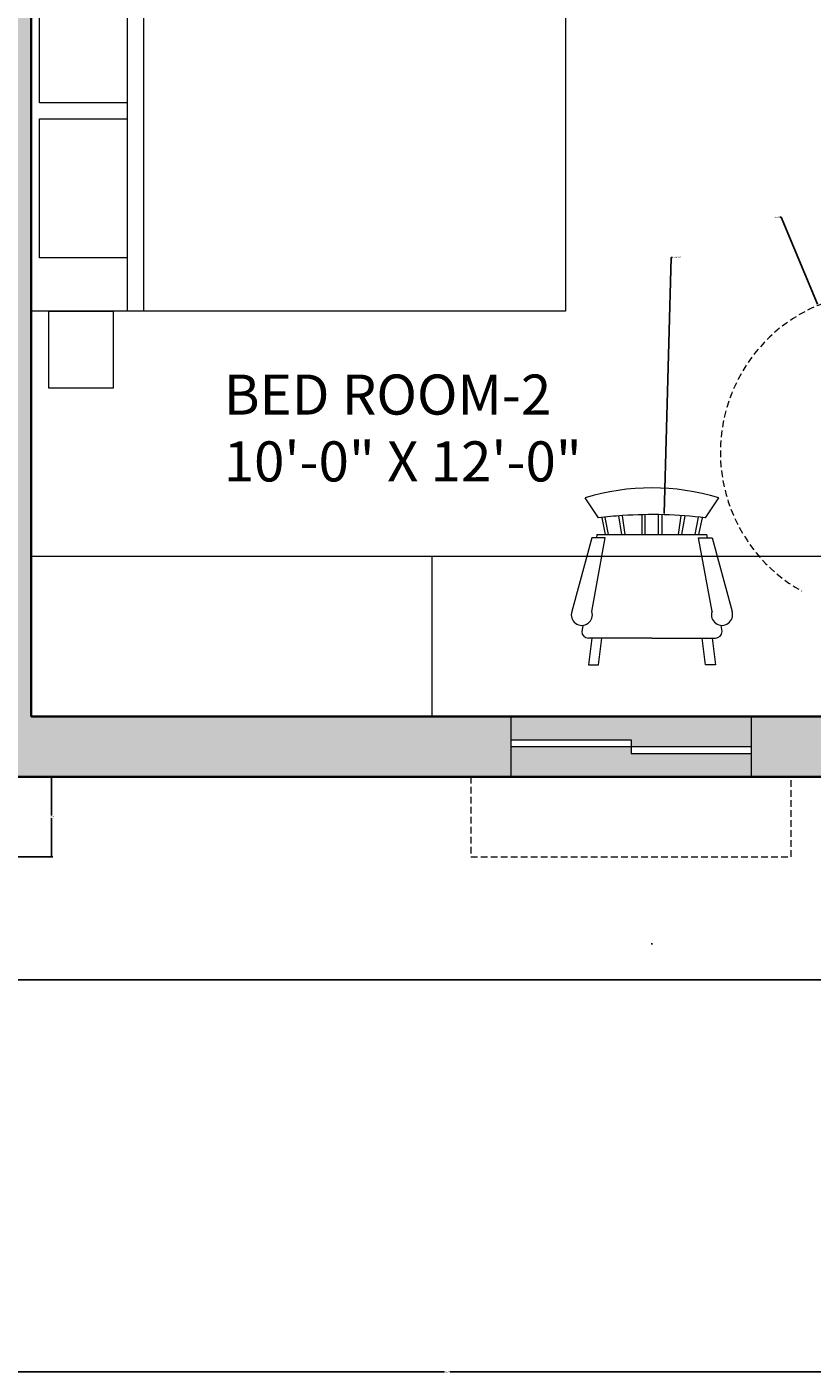
# Model space of a CAD drawing. Units: inches. Extents: x 1693 to 2974, y 2201 to 2965.
# Tile 8 of 24: x 1976 to 2093, y 2201 to 2402. Entities that reach past the tile are written whole.
import ezdxf

# ---------------------------------------------------------------- set-up
doc = ezdxf.new("R2010")
doc.units = ezdxf.units.IN
doc.header["$LTSCALE"] = 2
doc.header["$MEASUREMENT"] = 0
doc.linetypes.add('HIDDEN', pattern=[0.375, 0.25, -0.125])
for name, color, linetype, lineweight in [('A-ANNO-DIMS', 2, 'Continuous', 18), ('A-AREA-IDEN', 7, 'Continuous', 18), ('A-DOOR-SWNG', 3, 'HIDDEN', 13), ('A-FLOR-CASE', 32, 'Continuous', 18), ('A-FURN', 8, 'Continuous', 18), ('A-GLAZ', 4, 'Continuous', 18), ('A-GLAZ-OVHD', 8, 'HIDDEN', 13), ('A-WALL', 7, 'Continuous', 35)]:
    doc.layers.add(name, color=color, linetype=linetype, lineweight=lineweight)
doc.layers.add('A-GLAZ-PATT', color=141, linetype='Continuous', lineweight=13, true_color=0xadddf7)
doc.layers.add('A-WALL-PATT', color=251, linetype='Continuous', lineweight=13, true_color=0x636466)
doc.styles.get("Standard").update_dxf_attribs({"font": 'arial.ttf'})
doc.dimstyles.get("Standard").update_dxf_attribs({"dimtxt": 0.18, "dimasz": 0.18, "dimexe": 0.18, "dimexo": 0.0625, "dimgap": 0.09, "dimtad": 0, "dimtih": 1, "dimtoh": 1, "dimdec": 1, "dimzin": 0, "dimdsep": 46, "dimlunit": 3, "dimtxsty": 'Standard', "dimcen": 0.09, "dimadec": 0, "dimazin": 0, "dimtfac": 1, "dimtdec": 1, "dimtofl": 0, "dimtmove": 0, "dimatfit": 3, "dimfxl": 1, "dimtolj": 1, "dimtzin": 0, "dimarcsym": 0})

# ---------------------------------------------------------------- blocks, each defined once
blk = doc.blocks.new('Chair - Rocking')
for p, q in [((-8, -4.5), (-10, -1.5)), ((8, -4.5), (10, -1.5)), ((-7.5, -4.5), (-7, -7)), ((-6.5, -7), (-7.02225, -4.43)), ((-4.5, -7), (-4.96674, -4.19951)), ((-4, -7), (-4.40532, -4.16272)), ((-1.5, -4.05012), (-1.5, -7)), ((-1, -7), (-1, -4.05012)), ((1, -7), (1, -4.04655)), ((1.5, -4.05012), (1.5, -7)), ((4, -7), (4.40187, -4.18694)), ((4.5, -7), (4.96761, -4.19437)), ((6.5, -7), (7, -4.4057)), ((7.5, -4.5), (7, -7)), ((-9, -7.5), (-12, -18.49999)), ((-7, -7.5), (-9, -7.5)), ((-9, -18.49999), (-7, -7.5)), ((-8.23428, -6.99939), (-8.3093, -7.47958)), ((-8.23041, -7), (8.23915, -7)), ((7, -7.5), (9, -7.5)), ((9, -18.49999), (7, -7.5)), ((8.31071, -7.48854), (8.23449, -7.00073)), ((9, -7.5), (12, -18.49999)), ((-10.36644, -20.64523), (-10.5, -21.49999)), ((10.5, -21.49999), (10.3575, -20.58798)), ((-9, -22.49999), (-9.5, -26.49999)), ((0, -22.49999), (-9.5, -22.49999)), ((-8, -26.49999), (-7.5, -22.49999)), ((0, -22.49999), (9.5, -22.49999)), ((8, -26.49999), (7.5, -22.49999)), ((9, -22.49999), (9.5, -26.49999)), ((-9.5, -26.49999), (-8, -26.49999)), ((9.5, -26.49999), (8, -26.49999))]:
    blk.add_line(p, q)
for centre, radius, start, end in [((0, -34.08333), 34.08333, 72.93847, 107.0615), ((0, -68.25004), 64.25, 82.84733, 93.92211), ((0, -68.25004), 64.25, 93.92211, 97.15267), ((-10.5, -18.99999), 1.58114, 161.5651, 18.43495), ((10.5, -18.99999), 1.58114, 161.5651, 18.43495), ((-9.5, -21.49999), 1, 180, 270), ((9.5, -21.49999), 1, 270, 0)]:
    blk.add_arc(centre, radius, start, end)
blk = doc.blocks.new('Bed - Queen')
for p, q in [((0, -80.00003), (0, 0)), ((0, 0), (59.99999, 0)), ((59.99999, 0), (59.99999, -80.00003)), ((7.99999, -1.2), (28.79998, -1.2)), ((7.99999, -14.4), (7.99999, -1.2)), ((28.79998, -1.2), (28.79998, -14.4)), ((31.19999, -1.2), (51.99999, -1.2)), ((31.19999, -14.4), (31.19999, -1.2)), ((51.99999, -1.2), (51.99999, -16.4)), ((0, -14.4), (44.8, -14.4)), ((59.99999, -29.6), (44.8, -14.4)), ((44.8, -14.4), (44.8, -29.6)), ((44.8, -16.8), (0, -16.8)), ((51.99999, -16.4), (46.79936, -16.4)), ((44.8, -29.6), (59.99999, -29.6)), ((59.99999, -80.00003), (0, -80.00003))]:
    blk.add_line(p, q)
blk = doc.blocks.new('NIGHTSTAND')
at = {"ltscale": 2}
blk.add_lwpolyline([(11.51, 0), (0, 0), (0, 9.62), (11.51, 9.62)], close=True, dxfattribs=at)
blk = doc.blocks.new('WINDOW-HOOD-48IN')
at = {"ltscale": 2}
for p, q in [((12, 48), (0, 48)), ((0, 48), (0, 6)), ((12, 42), (12, 48)), ((0, 6), (0, 0)), ((0, 0), (12, 0))]:
    blk.add_line(p, q, dxfattribs=at)
blk = doc.blocks.new('*D52')
at = {"layer": 'A-ANNO-DIMS', "color": 0, "lineweight": -2, "ltscale": 2, "transparency": 16777216}
for p, q in [((1972.14, 2289.84), (1979.46, 2289.84)), ((1979.28, 2289.66), (1979.28, 2284.03)), ((1979.28, 2278.02), (1979.28, 2283.66)), ((1972.14, 2277.84), (1979.46, 2277.84))]:
    blk.add_line(p, q, dxfattribs=at)
at = {"layer": 'A-ANNO-DIMS', "color": 0, "ltscale": 2, "transparency": 16777216}
for points in [[(1979.25, 2289.66), (1979.31, 2289.66), (1979.28, 2289.84)], [(1979.25, 2278.02), (1979.31, 2278.02), (1979.28, 2277.84)]]:
    blk.add_solid(points, dxfattribs=at)
at = {"layer": 'Defpoints', "color": 0, "ltscale": 2, "transparency": 16777216}
for p in [(1972.08, 2289.84), (1979.28, 2289.84), (1972.08, 2277.84)]:
    blk.add_point(p, dxfattribs=at)
at = {"layer": 'A-ANNO-DIMS', "color": 0, "ltscale": 2, "transparency": 16777216, "insert": (1979.28, 2283.84), "char_height": 0.18, "attachment_point": 5}
blk.add_mtext('\\A1;12 TYP.', dxfattribs=at)
blk = doc.blocks.new('*D82')
at = {"layer": 'A-ANNO-DIMS', "color": 0, "lineweight": -2, "ltscale": 2, "transparency": 16777216}
for p, q in [((2615.67, 2906.08), (1693.46, 2906.08)), ((1693.64, 2905.9), (1693.64, 2582.94)), ((1693.64, 2259.62), (1693.64, 2582.58)), ((2096.17, 2259.44), (1693.46, 2259.44))]:
    blk.add_line(p, q, dxfattribs=at)
at = {"layer": 'A-ANNO-DIMS', "color": 0, "ltscale": 2, "transparency": 16777216}
for points in [[(1693.61, 2905.9), (1693.67, 2905.9), (1693.64, 2906.08)], [(1693.61, 2259.62), (1693.67, 2259.62), (1693.64, 2259.44)]]:
    blk.add_solid(points, dxfattribs=at)
at = {"layer": 'Defpoints', "color": 0, "ltscale": 2, "transparency": 16777216}
for p in [(1693.64, 2906.08), (2615.74, 2906.08), (2096.24, 2259.44)]:
    blk.add_point(p, dxfattribs=at)
at = {"layer": 'A-ANNO-DIMS', "color": 0, "ltscale": 2, "transparency": 16777216, "insert": (1693.64, 2582.76), "char_height": 0.18, "attachment_point": 5}
blk.add_mtext('\\A1;646.6', dxfattribs=at)
blk = doc.blocks.new('*D83')
at = {"layer": 'A-ANNO-DIMS', "color": 0, "lineweight": -2, "ltscale": 2, "transparency": 16777216}
for p, q in [((1782.74, 2289.78), (1782.74, 2200.56)), ((2294.24, 2289.78), (2294.24, 2200.56)), ((1782.92, 2200.74), (2038.09, 2200.74)), ((2294.06, 2200.74), (2038.88, 2200.74))]:
    blk.add_line(p, q, dxfattribs=at)
at = {"layer": 'A-ANNO-DIMS', "color": 0, "ltscale": 2, "transparency": 16777216}
for points in [[(1782.92, 2200.77), (1782.92, 2200.71), (1782.74, 2200.74)], [(2294.06, 2200.77), (2294.06, 2200.71), (2294.24, 2200.74)]]:
    blk.add_solid(points, dxfattribs=at)
at = {"layer": 'Defpoints', "color": 0, "ltscale": 2, "transparency": 16777216}
for p in [(1782.74, 2289.84), (2294.24, 2289.84), (2294.24, 2200.74)]:
    blk.add_point(p, dxfattribs=at)
at = {"layer": 'A-ANNO-DIMS', "color": 0, "ltscale": 2, "transparency": 16777216, "insert": (2038.49, 2200.74), "char_height": 0.18, "attachment_point": 5}
blk.add_mtext('\\A1;511.5', dxfattribs=at)
blk = doc.blocks.new('*D126')
at = {"layer": 'A-ANNO-DIMS', "color": 0, "lineweight": -2, "ltscale": 2, "transparency": 16777216}
for p, q in [((2088.31, 2373.6), (2088.49, 2373.6)), ((2088.49, 2373.6), (2093.95, 2360.58)), ((2103.15, 2338.43), (2103.33, 2338.43)), ((2103.24, 2338.34), (2103.24, 2338.52))]:
    blk.add_line(p, q, dxfattribs=at)
at = {"layer": 'A-ANNO-DIMS', "color": 0, "ltscale": 2, "transparency": 16777216}
blk.add_solid([(2093.98, 2360.59), (2093.93, 2360.57), (2094.02, 2360.41)], dxfattribs=at)
at = {"layer": 'Defpoints', "color": 0, "ltscale": 2, "transparency": 16777216}
for p in [(2094.02, 2360.41), (2103.24, 2338.43)]:
    blk.add_point(p, dxfattribs=at)
at = {"layer": 'A-ANNO-DIMS', "color": 0, "ltscale": 2, "transparency": 16777216, "insert": (2087.83, 2373.6), "char_height": 0.18, "attachment_point": 5}
blk.add_mtext('\\A1;R23.84', dxfattribs=at)
blk = doc.blocks.new('*D129')
at = {"layer": 'A-ANNO-DIMS', "color": 0, "lineweight": -2, "ltscale": 2, "transparency": 16777216}
for p, q in [((2072.05, 2367.59), (2070.97, 2329.24)), ((2072.23, 2367.59), (2072.05, 2367.59)), ((2069.06, 2264.83), (2069.24, 2264.83)), ((2069.15, 2264.74), (2069.15, 2264.92))]:
    blk.add_line(p, q, dxfattribs=at)
at = {"layer": 'A-ANNO-DIMS', "color": 0, "ltscale": 2, "transparency": 16777216}
blk.add_solid([(2070.94, 2329.24), (2071, 2329.24), (2070.96, 2329.06)], dxfattribs=at)
at = {"layer": 'Defpoints', "color": 0, "ltscale": 2, "transparency": 16777216}
for p in [(2070.96, 2329.06), (2069.15, 2264.83)]:
    blk.add_point(p, dxfattribs=at)
at = {"layer": 'A-ANNO-DIMS', "color": 0, "ltscale": 2, "transparency": 16777216, "insert": (2072.91, 2367.59), "char_height": 0.18, "attachment_point": 5}
blk.add_mtext('\\A1;4X R64.25', dxfattribs=at)

msp = doc.modelspace()

# ---------------------------------------------------------------- hatches: boundary and pattern name
at = {"layer": 'A-GLAZ-PATT', "ltscale": 2}
h = msp.add_hatch(color=256, dxfattribs=at)
h.dxf.hatch_style = 1
h.paths.add_polyline_path([(2656.9702, 2338.2547), (2632.9702, 2338.2547), (2632.9702, 2339.2547), (2608.9702, 2339.2547), (2608.9702, 2334.7547), (2656.9702, 2334.7547)])
h.paths.add_polyline_path([(2656.9702, 2343.7547), (2608.9702, 2343.7547), (2608.9702, 2340.2547), (2632.9702, 2340.2547), (2632.9702, 2339.2547), (2656.9702, 2339.2547)])
h.paths.add_polyline_path([(2775.7544, 2338.2547), (2751.7544, 2338.2547), (2751.7544, 2334.7547), (2775.7544, 2334.7547)])
h.paths.add_polyline_path([(2775.7544, 2343.7547), (2751.7544, 2343.7547), (2751.7544, 2340.2547), (2775.7544, 2340.2547)])
h.paths.add_polyline_path([(2897.7363, 2568.7999), (2893.2363, 2568.7999), (2893.2363, 2520.7999), (2896.7363, 2520.7999), (2896.7363, 2544.7999), (2897.7363, 2544.7999)])
h.paths.add_polyline_path([(2902.2363, 2568.7999), (2898.7363, 2568.7999), (2898.7363, 2544.7999), (2897.7363, 2544.7999), (2897.7363, 2520.7999), (2902.2363, 2520.7999)])
h.paths.add_polyline_path([(2902.2363, 2637.7547), (2898.7363, 2637.7547), (2898.7363, 2613.7547), (2902.2363, 2613.7547)])
h.paths.add_polyline_path([(2896.7363, 2637.7547), (2893.2363, 2637.7547), (2893.2363, 2613.7547), (2896.7363, 2613.7547)])
h.paths.add_polyline_path([(2902.2363, 2748.903), (2899.0477, 2748.903), (2899.0477, 2724.903), (2898.0477, 2724.903), (2898.0477, 2700.903), (2902.2363, 2700.903)])
h.paths.add_polyline_path([(2898.0477, 2748.903), (2893.2363, 2748.903), (2893.2363, 2700.903), (2897.0477, 2700.903), (2897.0477, 2724.903), (2898.0477, 2724.903)])
h.paths.add_polyline_path([(2851.2363, 2846.2547), (2803.2363, 2846.2547), (2803.2363, 2842.7547), (2827.2363, 2842.7547), (2827.2363, 2841.7547), (2851.2363, 2841.7547)])
h.paths.add_polyline_path([(2851.2363, 2840.7547), (2827.2363, 2840.7547), (2827.2363, 2841.7547), (2803.2363, 2841.7547), (2803.2363, 2837.2547), (2851.2363, 2837.2547)])
h.paths.add_polyline_path([(2578.2363, 2846.2547), (2530.2363, 2846.2547), (2530.2363, 2842.7547), (2554.2363, 2842.7547), (2554.2363, 2841.7547), (2578.2363, 2841.7547)])
h.paths.add_polyline_path([(2578.2363, 2840.7547), (2554.2363, 2840.7547), (2554.2363, 2841.7547), (2530.2363, 2841.7547), (2530.2363, 2837.2547), (2578.2363, 2837.2547)])
h.paths.add_polyline_path([(2732.7363, 2812.7547), (2705.1363, 2812.7547), (2705.1363, 2811.7547), (2676.3363, 2811.7547), (2676.3363, 2812.7547), (2648.7363, 2812.7547), (2648.7363, 2808.2547), (2732.7363, 2808.2547)])
h.paths.add_polyline_path([(2732.7363, 2817.2547), (2648.7363, 2817.2547), (2648.7363, 2813.7547), (2676.3363, 2813.7547), (2676.3363, 2812.7547), (2705.1363, 2812.7547), (2705.1363, 2813.7547), (2732.7363, 2813.7547)])
h.paths.add_polyline_path([(2488.2363, 2695.8203), (2484.7878, 2695.8203), (2484.7878, 2671.8203), (2488.2363, 2671.8203)])
h.paths.add_polyline_path([(2482.7878, 2695.8203), (2479.2363, 2695.8203), (2479.2363, 2671.8203), (2482.7878, 2671.8203)])
h.paths.add_polyline_path([(2488.2363, 2572.4371), (2484.7363, 2572.4371), (2484.7363, 2541.4371), (2483.7363, 2541.4371), (2483.7363, 2512.4371), (2488.2363, 2512.4371)])
h.paths.add_polyline_path([(2482.7363, 2541.4371), (2483.7363, 2541.4371), (2483.7363, 2572.4371), (2479.2363, 2572.4371), (2479.2363, 2512.4371), (2482.7363, 2512.4371)])
h.paths.add_polyline_path([(2248.9863, 2706.8449), (2190.9863, 2706.8449), (2190.9863, 2703.3449), (2219.9863, 2703.3449), (2219.9863, 2702.3449), (2248.9863, 2702.3449)])
h.paths.add_polyline_path([(2248.9863, 2701.3449), (2219.9863, 2701.3449), (2219.9863, 2702.3449), (2190.9863, 2702.3449), (2190.9863, 2697.8449), (2248.9863, 2697.8449)])
h.paths.add_polyline_path([(2151.9207, 2293.3449), (2127.9207, 2293.3449), (2127.9207, 2289.8449), (2151.9207, 2289.8449)])
h.paths.add_polyline_path([(2151.9207, 2298.8449), (2127.9207, 2298.8449), (2127.9207, 2295.3449), (2151.9207, 2295.3449)])
h.paths.add_polyline_path([(2084.023, 2293.3449), (2066.023, 2293.3449), (2066.023, 2294.3449), (2048.023, 2294.3449), (2048.023, 2289.8449), (2084.023, 2289.8449)])
h.paths.add_polyline_path([(2084.023, 2298.8449), (2048.023, 2298.8449), (2048.023, 2295.3449), (2066.023, 2295.3449), (2066.023, 2294.3449), (2084.023, 2294.3449)])
h.paths.add_polyline_path([(1966.0781, 2293.3449), (1948.0781, 2293.3449), (1948.0781, 2294.3449), (1930.0781, 2294.3449), (1930.0781, 2289.8449), (1966.0781, 2289.8449)])
h.paths.add_polyline_path([(1966.0781, 2298.8449), (1930.0781, 2298.8449), (1930.0781, 2295.3449), (1948.0781, 2295.3449), (1948.0781, 2294.3449), (1966.0781, 2294.3449)])
h.paths.add_polyline_path([(1787.2363, 2403.1922), (1782.7363, 2403.1922), (1782.7363, 2355.1922), (1786.2363, 2355.1922), (1786.2363, 2379.1922), (1787.2363, 2379.1922)])
h.paths.add_polyline_path([(1791.7363, 2403.1922), (1788.2363, 2403.1922), (1788.2363, 2379.1922), (1787.2363, 2379.1922), (1787.2363, 2355.1922), (1791.7363, 2355.1922)])
h.paths.add_polyline_path([(1786.2363, 2477.5455), (1782.7363, 2477.5455), (1782.7363, 2453.5455), (1786.2363, 2453.5455)])
h.paths.add_polyline_path([(1791.7363, 2477.5455), (1788.2363, 2477.5455), (1788.2363, 2453.5455), (1791.7363, 2453.5455)])
h.paths.add_polyline_path([(1786.2363, 2621.6433), (1782.7363, 2621.6433), (1782.7363, 2585.6433), (1786.2363, 2585.6433)])
h.paths.add_polyline_path([(1791.7363, 2621.6433), (1788.2363, 2621.6433), (1788.2363, 2585.6433), (1791.7363, 2585.6433)])
h.paths.add_polyline_path([(1908.1286, 2706.8449), (1860.1286, 2706.8449), (1860.1286, 2703.3449), (1884.1286, 2703.3449), (1884.1286, 2702.3449), (1908.1286, 2702.3449)])
h.paths.add_polyline_path([(1908.1286, 2701.3449), (1884.1286, 2701.3449), (1884.1286, 2702.3449), (1860.1286, 2702.3449), (1860.1286, 2697.8449), (1908.1286, 2697.8449)])
h.paths.add_polyline_path([(1973.9863, 2706.8449), (1949.9863, 2706.8449), (1949.9863, 2703.3449), (1973.9863, 2703.3449)])
h.paths.add_polyline_path([(1973.9863, 2701.3449), (1949.9863, 2701.3449), (1949.9863, 2697.8449), (1973.9863, 2697.8449)])
h.paths.add_polyline_path([(2112.7363, 2690.3449), (2028.7363, 2690.3449), (2028.7363, 2686.8449), (2056.3363, 2686.8449), (2056.3363, 2685.8449), (2085.1363, 2685.8449), (2085.1363, 2686.8449), (2112.7363, 2686.8449)])
h.paths.add_polyline_path([(2112.7363, 2685.8449), (2085.1363, 2685.8449), (2085.1363, 2684.8449), (2056.3363, 2684.8449), (2056.3363, 2685.8449), (2028.7363, 2685.8449), (2028.7363, 2681.3449), (2112.7363, 2681.3449)])
h.paths.add_polyline_path([(2422.7363, 2640.7547), (2350.7363, 2640.7547), (2350.7363, 2637.2547), (2386.7363, 2637.2547), (2386.7363, 2636.2547), (2422.7363, 2636.2547)])
h.paths.add_polyline_path([(2422.7363, 2635.2547), (2386.7363, 2635.2547), (2386.7363, 2636.2547), (2350.7363, 2636.2547), (2350.7363, 2631.7547), (2422.7363, 2631.7547)])
at = {"layer": 'A-WALL-PATT', "ltscale": 2}
h = msp.add_hatch(color=256, dxfattribs=at)
h.dxf.hatch_style = 1
h.paths.add_polyline_path([(2294.2363, 2706.8449), (2248.9863, 2706.8449), (2248.9863, 2697.8449), (2285.2363, 2697.8449), (2285.2363, 2586.2648), (2294.2363, 2586.2648)])
h.paths.add_polyline_path([(2294.2363, 2550.2648), (2285.2363, 2550.2648), (2285.2363, 2517.8449), (2141.2363, 2517.8449), (2141.2363, 2513.8449), (2285.2363, 2513.8449), (2285.2363, 2369.8449), (2253.0704, 2369.8449), (2253.0704, 2366.8449), (2285.2363, 2366.8449), (2285.2363, 2298.8449), (2165.2363, 2298.8449), (2165.2363, 2366.8449), (2165.2363, 2369.8449), (2165.2363, 2447.3449), (2160.7363, 2447.3449), (2160.7363, 2403.3449), (2100.7363, 2403.3449), (2100.7363, 2447.3449), (2094.2363, 2447.3449), (2094.2363, 2442.8449), (2096.2363, 2442.8449), (2096.2363, 2362.1344), (2100.7363, 2362.1344), (2100.7363, 2400.8449), (2160.7363, 2400.8449), (2160.7363, 2298.8449), (2151.9207, 2298.8449), (2151.9207, 2289.8449), (2184.7363, 2289.8449), (2184.7363, 2276.6449), (2189.2363, 2276.6449), (2189.2363, 2289.8449), (2294.2363, 2289.8449)])
h.paths.add_polyline_path([(2048.023, 2298.8449), (1976.2363, 2298.8449), (1976.2363, 2442.8449), (2058.2363, 2442.8449, -0.00822734), (2058.2363, 2443.9061), (2058.2363, 2447.3449), (2004.7363, 2447.3449), (1969.7363, 2447.3449), (1969.7363, 2442.8449), (1971.7363, 2442.8449), (1971.7363, 2298.8449), (1966.0781, 2298.8449), (1966.0781, 2289.8449), (2048.023, 2289.8449)])
h.paths.add_polyline_path([(2127.9207, 2298.8449), (2100.7363, 2298.8449), (2100.7363, 2332.1344), (2096.2363, 2332.1344), (2096.2363, 2298.8449), (2084.023, 2298.8449), (2084.023, 2289.8449), (2096.2363, 2289.8449), (2096.2363, 2259.4449), (2114.3201, 2259.4449), (2114.3201, 2263.4449), (2100.7363, 2263.4449), (2100.7363, 2289.8449), (2127.9207, 2289.8449)])

# ---------------------------------------------------------------- linework, layer by layer
at = {"layer": 'A-DOOR-SWNG', "ltscale": 2}
msp.add_arc((2103.2428, 2338.4274), 23.8391, 344.693751, 240.808744, dxfattribs=at)
at = {"layer": 'A-FLOR-CASE'}
msp.add_line((1976.2363, 2322.8449), (2096.2363, 2322.8449), dxfattribs=at)
at = {"layer": 'A-FLOR-CASE', "ltscale": 2}
msp.add_line((2036.2363, 2298.8449), (2036.2363, 2322.8449), dxfattribs=at)
at = {"layer": 'A-GLAZ', "ltscale": 2}
for p, q in [((2048.023, 2298.8449), (2048.023, 2289.8449)), ((2084.023, 2298.8449), (2084.023, 2289.8449)), ((2048.023, 2295.3449), (2066.023, 2295.3449)), ((2048.023, 2294.3449), (2084.023, 2294.3449)), ((2066.023, 2295.3449), (2066.023, 2293.3449)), ((2066.023, 2293.3449), (2084.023, 2293.3449))]:
    msp.add_line(p, q, dxfattribs=at)
at = {"layer": 'A-WALL'}
for p, q in [((1976.2363, 2442.8449), (1976.2363, 2298.8449)), ((1976.2363, 2298.8449), (2096.2363, 2298.8449)), ((1782.7363, 2289.8449), (2096.2363, 2289.8449))]:
    msp.add_line(p, q, dxfattribs=at)

# ---------------------------------------------------------------- block references
at = {"layer": 'A-FURN', "ltscale": 2, "rotation": 89.99999999999999}
msp.add_blockref('Bed - Queen', (1976.2363, 2359.5424), dxfattribs=at)
at = {"layer": 'A-FURN', "rotation": 270.0000000000013}
msp.add_blockref('NIGHTSTAND', (1978.8504, 2359.5424), dxfattribs=at)
at = {"layer": 'A-FURN', "ltscale": 2}
msp.add_blockref('Chair - Rocking', (2069.1495, 2333.085), dxfattribs=at)
at = {"layer": 'A-GLAZ-OVHD', "rotation": 90.0000000000003}
msp.add_blockref('WINDOW-HOOD-48IN', (2090.0233, 2277.8446), dxfattribs=at)

# ---------------------------------------------------------------- texts
at = {"layer": 'A-AREA-IDEN', "ltscale": 2, "insert": (2005.04, 2350.0507), "char_height": 6, "attachment_point": 1}
msp.add_mtext_dynamic_manual_height_columns('BED ROOM-2\\P10\'-0" X 12\'-0"', width=108.452746, gutter_width=1, heights=[0], dxfattribs=at)

# ---------------------------------------------------------------- dimensions: what is measured, and where the dimension line sits
at = {"layer": 'A-ANNO-DIMS', "ltscale": 2}
dim = msp.add_linear_dim(base=(1693.6363, 2906.0761), p1=(2096.2363, 2259.4449), p2=(2615.7363, 2906.0761), angle=90, dimstyle='Standard', override={"dimdec": 1, "dimlfac": 1, "dimrnd": 0, "dimzin": 0, "dimdsep": 46, "dimlunit": 2}, dxfattribs=at)
dim.commit()
dim.dimension.update_dxf_attribs({"geometry": '*D82', "text_midpoint": (1693.6363, 2582.7605)})
dim = msp.add_radius_dim(center=(2103.2428, 2338.4274), mpoint=(2094.0232, 2360.4116), dimstyle='Standard', override={"dimdec": 2, "dimlfac": 1, "dimrnd": 0, "dimzin": 0, "dimdsep": 46, "dimlunit": 2}, dxfattribs=at)
dim.commit()
dim.dimension.update_dxf_attribs({"geometry": '*D126', "text_midpoint": (2087.8319, 2373.6021), "dimtype": 164})
dim = msp.add_radius_dim(center=(2069.1495, 2264.8349), mpoint=(2070.961, 2329.0594), text='4X <>', dimstyle='Standard', override={"dimdec": 2, "dimlfac": 1, "dimrnd": 0, "dimzin": 0, "dimdsep": 46, "dimlunit": 2}, dxfattribs=at)
dim.commit()
dim.dimension.update_dxf_attribs({"geometry": '*D129', "text_midpoint": (2072.9055, 2367.5941), "dimtype": 164})
dim = msp.add_linear_dim(base=(2294.2363, 2200.7449), p1=(1782.7363, 2289.8449), p2=(2294.2363, 2289.8449), dimstyle='Standard', override={"dimdec": 1, "dimlfac": 1, "dimrnd": 0, "dimzin": 0, "dimdsep": 46, "dimlunit": 2}, dxfattribs=at)
dim.commit()
dim.dimension.update_dxf_attribs({"geometry": '*D83', "text_midpoint": (2038.4863, 2200.7449)})
dim = msp.add_linear_dim(base=(1979.2781, 2289.8449), p1=(1972.0781, 2277.8449), p2=(1972.0781, 2289.8449), angle=90, text='<> TYP.', dimstyle='Standard', override={"dimdec": 0, "dimlfac": 1, "dimrnd": 0, "dimzin": 0, "dimdsep": 46, "dimlunit": 2}, dxfattribs=at)
dim.commit()
dim.dimension.update_dxf_attribs({"geometry": '*D52', "text_midpoint": (1979.2781, 2283.8449)})

doc.saveas('drawing.dxf')
